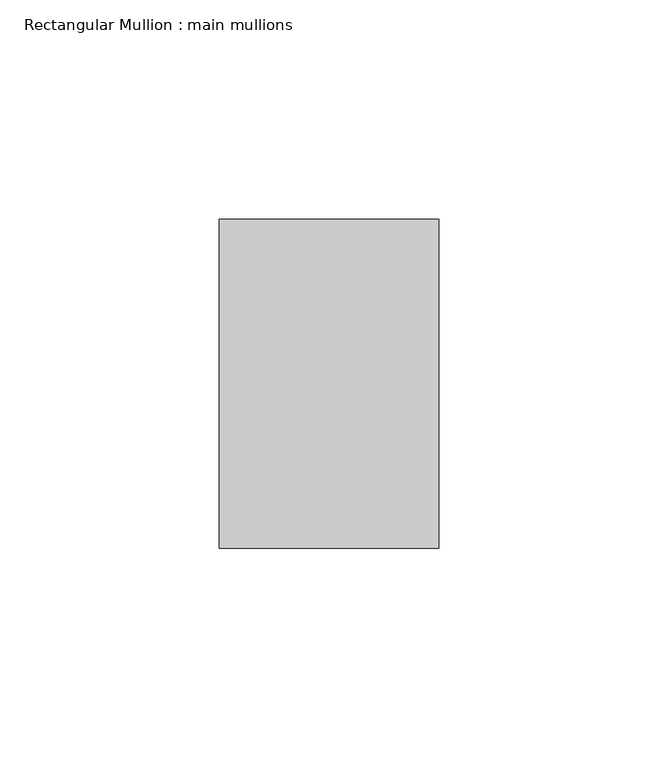
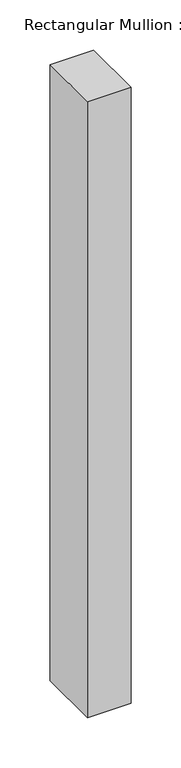
"""IFC4 building model written with IfcOpenShell, lengths in millimetres: member geometry, Rectangular Mullion : main mullions."""

from ifc_helpers import new_model, si_unit, frame, origin, place, context, project, spatial, polyline, outline, extrude, source, transform, mapped, element, save


def rectangular_mullion_main_mullions_65d9d1a0(model_context):
    return source(origin(), model_context, "Body", "SweptSolid", [
        extrude(outline(polyline([(0.0, 37.5), (0.0, -37.5), (-50.0, -37.5), (-50.0, 37.5), (0.0, 37.5)])), frame((0.0, 0.0, -750.0), z_axis=(0.0, 0.0, 1.0), x_axis=(1.0, 0.0, 0.0)), (0.0, 0.0, 1.0), 750.0),
    ])


if __name__ == "__main__":
    model = new_model("IFC4")
    model_context = context("Model", 3, world=origin())
    ifc_project = project(units=[si_unit("LENGTHUNIT", "METRE", prefix="MILLI")], contexts=[model_context])
    site = spatial("IfcSite", under=ifc_project)
    building = spatial("IfcBuilding", under=site)
    placement = place(None, origin())
    rectangular_mullion_main_mullions_shape = rectangular_mullion_main_mullions_65d9d1a0(model_context)
    element("IfcMember", 1, ObjectType="Rectangular Mullion : main mullions", at=placement, inside=building, context=model_context, shape_type="MappedRepresentation", body=[
        mapped(rectangular_mullion_main_mullions_shape, transform((0.0, 0.0, 0.0), x_axis=(1.0, 0.0, 0.0), y_axis=(0.0, 1.0, 0.0), z_axis=(0.0, 0.0, 1.0))),
    ])
    save(model, "model.ifc")

# Revit data of these elements
# Type "Rectangular Mullion : main mullions"
#   built-in parameter 1007304 = 0.246063 (stored number, unit not read)
#   built-in parameter 1007301 = 0.082021 (stored number, unit not read)
#   built-in parameter 1007300 = 0.082021 (stored number, unit not read)
# Element 1 (IfcMember, "Rectangular Mullion : main mullions")
#   Materials on its faces: "Aluminum"
# Materials
#   "Aluminum": class "Metal", colour RGB 136 136 136, transparency 0, Description = "Aluminum 6061", Cost = 0
